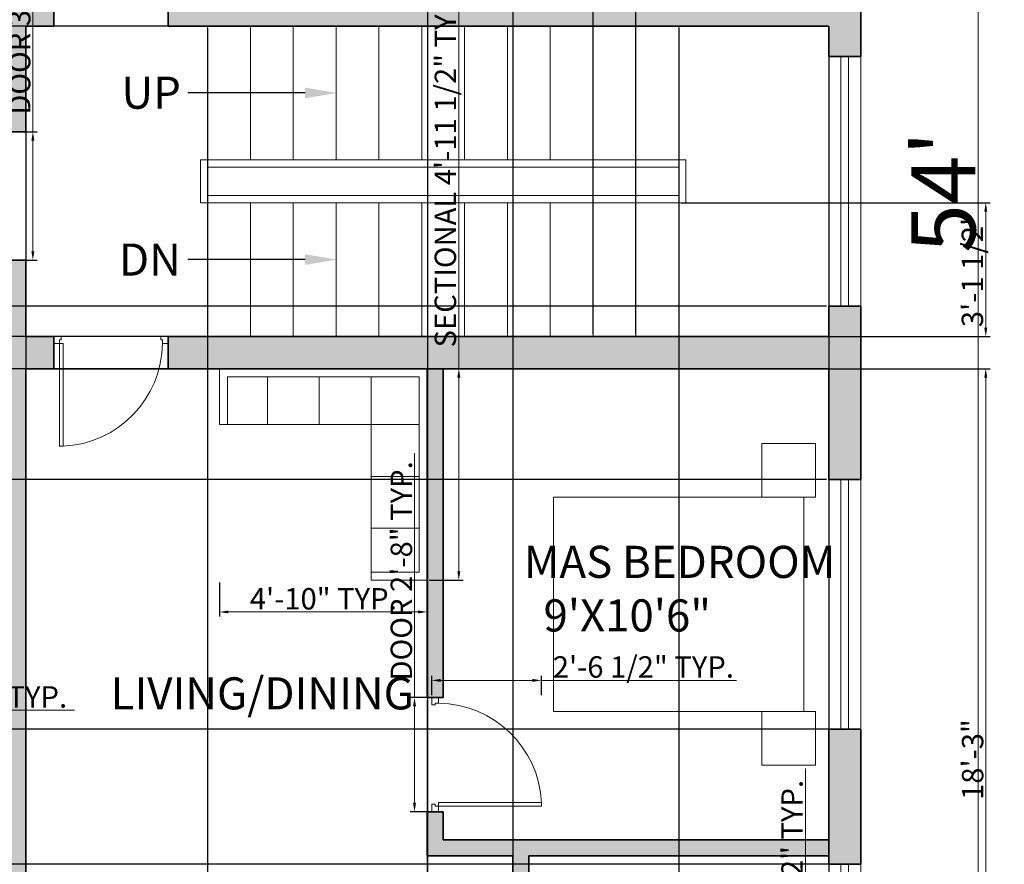
# Model space of a CAD drawing. Units: inches. Extents: x 2696 to 3240, y 1564 to 2310.
# Tile 38 of 76: x 2964 to 3240, y 1745 to 1982. Entities that reach past the tile are written whole.
import ezdxf
from ezdxf import colors
from ezdxf.entities.mleader import LeaderData, LeaderLine
from ezdxf.math import Vec2, Vec3

# ---------------------------------------------------------------- set-up
doc = ezdxf.new("R2010")
doc.units = ezdxf.units.IN
for name, color, linetype, lineweight in [('A-ANNO-DIMS', 3, 'Continuous', 18), ('A-ANNO-SYMB', 7, 'Continuous', 18), ('A-AREA-IDEN', 7, 'Continuous', 18), ('A-DOOR', 4, 'Continuous', 18), ('A-FLOR-STRS', 7, 'Continuous', 18), ('A-FURN', 251, 'Continuous', 13), ('A-WALL', 7, 'Continuous', 35), ('A-WALL-PATT', 9, 'Continuous', 13), ('WINDOW', 2, 'Continuous', 18)]:
    doc.layers.add(name, color=color, linetype=linetype, lineweight=lineweight)
doc.styles.get("Standard").update_dxf_attribs({"font": 'arial.ttf'})
doc.styles.add('TIMES NEW', font='times.ttf')
doc.styles.add('YQ_DIM', font='SUPEROS.SHX', dxfattribs={"width": 0.8, "bigfont": 'HZDX.SHX'})
doc.dimstyles.new('Siddhuu', dxfattribs={"dimtxt": 6, "dimasz": 2.5, "dimexe": 1.25, "dimexo": 0.625, "dimtad": 1, "dimdec": 1, "dimlunit": 4, "dimtxsty": 'TIMES NEW', "dimcen": 2.5, "dimclrd": 256, "dimclre": 1, "dimclrt": 7, "dimadec": 0, "dimazin": 0, "dimtfac": 1, "dimtdec": 1, "dimtmove": 0, "dimatfit": 3, "dimfxl": 1, "dimtolj": 1, "dimlwd": -1, "dimarcsym": 0})

# ---------------------------------------------------------------- blocks, each defined once
blk = doc.blocks.new('DR_D01')
for p, q in [((-0.45, 0.93), (-0.42, 0.93)), ((-0.45, 0.03), (-0.45, 0.93)), ((-0.42, 0.03), (-0.42, 0.93)), ((-0.5, 0.03), (-0.42, 0.03)), ((-0.5, 0.03), (-0.5, -0.03)), ((-0.45, 0.03), (-0.45, 0)), ((-0.45, 0), (-0.435, 0)), ((-0.435, 0), (-0.435, -0.03)), ((0.435, 0), (0.435, -0.03)), ((0.45, 0), (0.435, 0)), ((0.45, 0.03), (0.45, 0)), ((0.5, 0.03), (0.45, 0.03)), ((0.5, -0.03), (0.5, 0.03)), ((-0.435, -0.03), (-0.5, -0.03)), ((0.435, -0.03), (0.5, -0.03))]:
    blk.add_line(p, q)
blk.add_arc((-0.4602, 0.0206), 0.9103, 0.59152, 87.46644)
blk = doc.blocks.new('WD_WIN4')
for p, q in [((-0.5, 0.5), (0.5, 0.5)), ((-0.5, 0.12), (0.5, 0.12)), ((-0.5, -0.12), (0.5, -0.12)), ((-0.5, -0.5), (0.5, -0.5))]:
    blk.add_line(p, q)
blk = doc.blocks.new('*D10')
at = {"layer": 'A-ANNO-DIMS', "color": 0, "lineweight": -2, "transparency": 16777216}
for p, q in [((3200.24, 2262.2), (3233.75, 2262.2)), ((3200.24, 1605.2), (3233.75, 1605.2))]:
    blk.add_line(p, q, dxfattribs=at)
at = {"layer": 'A-ANNO-DIMS', "color": 0, "transparency": 16777216}
blk.add_line((3232.5, 2250.2), (3232.5, 1617.2), dxfattribs=at)
for points in [[(3230.5, 2250.2), (3234.5, 2250.2), (3232.5, 2262.2)], [(3230.5, 1617.2), (3234.5, 1617.2), (3232.5, 1605.2)]]:
    blk.add_solid(points, dxfattribs=at)
at = {"layer": 'Defpoints', "color": 0, "transparency": 16777216}
for p in [(3199.61, 2262.2), (3199.61, 1605.2), (3232.5, 1605.2)]:
    blk.add_point(p, dxfattribs=at)
at = {"layer": 'A-ANNO-DIMS', "color": 0, "transparency": 16777216, "insert": (3222.71, 1933.7), "char_height": 18, "attachment_point": 5, "rotation": 90, "style": 'TIMES NEW'}
blk.add_mtext("\\A1;54'", dxfattribs=at)
blk = doc.blocks.new('BED-DOUBLE-WITH-NIGHTSTANDS')
for points in [[(0, 75.13), (0, 90.16), (15.03, 90.16), (15.03, 75.13)], [(3.28, 15.03), (3.28, 75.13), (73.4, 75.13), (73.4, 15.03)], [(0, 15.03), (0, 0), (15.03, 0), (15.03, 15.03)]]:
    blk.add_lwpolyline(points, close=True)
blk = doc.blocks.new('SOFA-SECTIONAL')
for p, q in [((0, 43.61), (0, 59.26)), ((0, 59.26), (58.14, 59.26)), ((58.14, 59.26), (58.14, 0)), ((2.24, 43.61), (2.24, 57.02)), ((2.24, 57.02), (55.9, 57.02)), ((13.42, 57.02), (13.42, 43.61)), ((27.95, 57.02), (27.95, 43.61)), ((42.49, 57.02), (42.49, 0)), ((55.9, 57.02), (55.9, 2.24)), ((0, 43.61), (55.9, 43.61)), ((42.49, 29.07), (55.9, 29.07)), ((42.49, 14.54), (55.9, 14.54)), ((55.9, 2.24), (42.49, 2.24)), ((58.14, 0), (42.49, 0))]:
    blk.add_line(p, q)
blk = doc.blocks.new('*D26')
at = {"layer": 'A-ANNO-DIMS', "transparency": 16777216}
for p, q in [((3184.12, 1676.35), (3184.12, 1772.17)), ((3184.12, 1635.55), (3184.12, 1673.85))]:
    blk.add_line(p, q, dxfattribs=at)
at = {"layer": 'A-ANNO-DIMS', "color": 1, "lineweight": -2, "transparency": 16777216}
for p, q in [((3189.99, 1676.35), (3182.87, 1676.35)), ((3189.99, 1633.05), (3182.87, 1633.05))]:
    blk.add_line(p, q, dxfattribs=at)
at = {"layer": 'A-ANNO-DIMS', "transparency": 16777216}
for points in [[(3183.7, 1673.85), (3184.53, 1673.85), (3184.12, 1676.35)], [(3183.7, 1635.55), (3184.53, 1635.55), (3184.12, 1633.05)]]:
    blk.add_solid(points, dxfattribs=at)
at = {"layer": 'Defpoints', "color": 0, "transparency": 16777216}
for p in [(3184.12, 1676.35), (3190.61, 1676.35), (3190.61, 1633.05)]:
    blk.add_point(p, dxfattribs=at)
at = {"layer": 'A-ANNO-DIMS', "color": 7, "transparency": 16777216, "insert": (3180.35, 1725.51), "char_height": 6, "attachment_point": 5, "rotation": 90, "style": 'TIMES NEW'}
blk.add_mtext('\\A1;WINDOW 3\'-7 1/2" TYP.', dxfattribs=at)
blk = doc.blocks.new('*D30')
at = {"layer": 'A-ANNO-DIMS', "transparency": 16777216}
for p, q in [((2967.69, 1950.58), (2967.69, 2019.05)), ((2967.69, 1917.08), (2967.69, 1948.08))]:
    blk.add_line(p, q, dxfattribs=at)
at = {"layer": 'A-ANNO-DIMS', "color": 1, "lineweight": -2, "transparency": 16777216}
for p, q in [((2962.91, 1950.58), (2968.94, 1950.58)), ((2962.91, 1914.58), (2968.94, 1914.58))]:
    blk.add_line(p, q, dxfattribs=at)
at = {"layer": 'A-ANNO-DIMS', "transparency": 16777216}
for points in [[(2967.27, 1948.08), (2968.11, 1948.08), (2967.69, 1950.58)], [(2967.27, 1917.08), (2968.11, 1917.08), (2967.69, 1914.58)]]:
    blk.add_solid(points, dxfattribs=at)
at = {"layer": 'Defpoints', "color": 0, "transparency": 16777216}
for p in [(2962.29, 1950.58), (2967.69, 1950.58), (2962.29, 1914.58)]:
    blk.add_point(p, dxfattribs=at)
at = {"layer": 'A-ANNO-DIMS', "color": 7, "transparency": 16777216, "insert": (2964, 1986.06), "char_height": 6, "attachment_point": 5, "rotation": 90, "style": 'TIMES NEW'}
blk.add_mtext('\\A1;DOOR 3\'-0" TYP.', dxfattribs=at)
blk = doc.blocks.new('*D34')
at = {"layer": 'A-ANNO-DIMS', "transparency": 16777216}
for p, q in [((3074.6, 1792.08), (3074.6, 1860.55)), ((3074.6, 1762.58), (3074.6, 1789.58))]:
    blk.add_line(p, q, dxfattribs=at)
at = {"layer": 'A-ANNO-DIMS', "color": 1, "lineweight": -2, "transparency": 16777216}
for p, q in [((3078.78, 1792.08), (3073.35, 1792.08)), ((3078.78, 1760.08), (3073.35, 1760.08))]:
    blk.add_line(p, q, dxfattribs=at)
at = {"layer": 'A-ANNO-DIMS', "transparency": 16777216}
for points in [[(3074.18, 1789.58), (3075.02, 1789.58), (3074.6, 1792.08)], [(3074.18, 1762.58), (3075.02, 1762.58), (3074.6, 1760.08)]]:
    blk.add_solid(points, dxfattribs=at)
at = {"layer": 'Defpoints', "color": 0, "transparency": 16777216}
for p in [(3074.6, 1792.08), (3079.4, 1792.08), (3079.4, 1760.08)]:
    blk.add_point(p, dxfattribs=at)
at = {"layer": 'A-ANNO-DIMS', "color": 7, "transparency": 16777216, "insert": (3070.91, 1827.56), "char_height": 6, "attachment_point": 5, "rotation": 90, "style": 'TIMES NEW'}
blk.add_mtext('\\A1;DOOR 2\'-8" TYP.', dxfattribs=at)
blk = doc.blocks.new('*D35')
at = {"layer": 'A-ANNO-DIMS', "color": 1, "lineweight": -2, "transparency": 16777216}
for p, q in [((3079.4, 1792.7), (3079.4, 1798.13)), ((3110.12, 1792.7), (3110.12, 1798.13))]:
    blk.add_line(p, q, dxfattribs=at)
at = {"layer": 'A-ANNO-DIMS', "transparency": 16777216}
for p, q in [((3081.9, 1796.88), (3107.62, 1796.88)), ((3110.12, 1796.88), (3164.78, 1796.88))]:
    blk.add_line(p, q, dxfattribs=at)
for points in [[(3081.9, 1797.29), (3081.9, 1796.46), (3079.4, 1796.88)], [(3107.62, 1797.29), (3107.62, 1796.46), (3110.12, 1796.88)]]:
    blk.add_solid(points, dxfattribs=at)
at = {"layer": 'Defpoints', "color": 0, "transparency": 16777216}
for p in [(3110.12, 1796.88), (3079.4, 1792.08), (3110.12, 1792.08)]:
    blk.add_point(p, dxfattribs=at)
at = {"layer": 'A-ANNO-DIMS', "color": 7, "transparency": 16777216, "insert": (3138.7, 1800.64), "char_height": 6, "attachment_point": 5, "style": 'TIMES NEW'}
blk.add_mtext('\\A1;2\'-6 1/2" TYP.', dxfattribs=at)
blk = doc.blocks.new('*D42')
at = {"layer": 'A-ANNO-DIMS', "color": 1, "lineweight": -2, "transparency": 16777216}
for p, q in [((2884.71, 1792.59), (2884.71, 1787.31)), ((2915.75, 1792.59), (2915.75, 1787.31))]:
    blk.add_line(p, q, dxfattribs=at)
at = {"layer": 'A-ANNO-DIMS', "transparency": 16777216}
for p, q in [((2887.21, 1788.56), (2913.25, 1788.56)), ((2915.75, 1788.56), (2979.39, 1788.56))]:
    blk.add_line(p, q, dxfattribs=at)
for points in [[(2887.21, 1788.98), (2887.21, 1788.14), (2884.71, 1788.56)], [(2913.25, 1788.98), (2913.25, 1788.14), (2915.75, 1788.56)]]:
    blk.add_solid(points, dxfattribs=at)
at = {"layer": 'Defpoints', "color": 0, "transparency": 16777216}
for p in [(2884.71, 1793.22), (2915.75, 1793.22), (2915.75, 1788.56)]:
    blk.add_point(p, dxfattribs=at)
at = {"layer": 'A-ANNO-DIMS', "color": 7, "transparency": 16777216, "insert": (2948.82, 1792.25), "char_height": 6, "attachment_point": 5, "style": 'TIMES NEW'}
blk.add_mtext('\\A1;SINK 2\'-7" TYP.', dxfattribs=at)
blk = doc.blocks.new('*D48')
at = {"layer": 'A-ANNO-DIMS', "transparency": 16777216}
for p, q in [((3087, 1884.2), (3087, 1994.35)), ((3087, 1827.44), (3087, 1881.7))]:
    blk.add_line(p, q, dxfattribs=at)
at = {"layer": 'A-ANNO-DIMS', "color": 1, "lineweight": -2, "transparency": 16777216}
for p, q in [((3078.74, 1884.2), (3088.25, 1884.2)), ((3078.74, 1824.94), (3088.25, 1824.94))]:
    blk.add_line(p, q, dxfattribs=at)
at = {"layer": 'A-ANNO-DIMS', "transparency": 16777216}
for points in [[(3086.58, 1881.7), (3087.42, 1881.7), (3087, 1884.2)], [(3086.58, 1827.44), (3087.42, 1827.44), (3087, 1824.94)]]:
    blk.add_solid(points, dxfattribs=at)
at = {"layer": 'Defpoints', "color": 0, "transparency": 16777216}
for p in [(3078.11, 1884.2), (3087, 1884.2), (3078.11, 1824.94)]:
    blk.add_point(p, dxfattribs=at)
at = {"layer": 'A-ANNO-DIMS', "color": 7, "transparency": 16777216, "insert": (3083.23, 1940.53), "char_height": 6, "attachment_point": 5, "rotation": 90, "style": 'TIMES NEW'}
blk.add_mtext('\\A1;SECTIONAL 4\'-11 1/2" TYP.', dxfattribs=at)
blk = doc.blocks.new('*D49')
at = {"layer": 'A-ANNO-DIMS', "color": 1, "lineweight": -2, "transparency": 16777216}
for p, q in [((3019.97, 1824.32), (3019.97, 1814.8)), ((3078.11, 1824.32), (3078.11, 1814.8))]:
    blk.add_line(p, q, dxfattribs=at)
at = {"layer": 'A-ANNO-DIMS', "transparency": 16777216}
blk.add_line((3022.47, 1816.05), (3075.61, 1816.05), dxfattribs=at)
for points in [[(3022.47, 1816.47), (3022.47, 1815.64), (3019.97, 1816.05)], [(3075.61, 1816.47), (3075.61, 1815.64), (3078.11, 1816.05)]]:
    blk.add_solid(points, dxfattribs=at)
at = {"layer": 'Defpoints', "color": 0, "transparency": 16777216}
for p in [(3019.97, 1824.94), (3078.11, 1824.94), (3078.11, 1816.05)]:
    blk.add_point(p, dxfattribs=at)
at = {"layer": 'A-ANNO-DIMS', "color": 7, "transparency": 16777216, "insert": (3049.04, 1819.74), "char_height": 6, "attachment_point": 5, "style": 'TIMES NEW'}
blk.add_mtext('\\A1;4\'-10" TYP.', dxfattribs=at)
blk = doc.blocks.new('*D50')
at = {"layer": 'A-ANNO-DIMS', "color": 1, "lineweight": -2, "transparency": 16777216}
for p, q in [((2965.71, 1979.58), (2965.71, 1568.95)), ((3016.61, 1979.58), (3016.61, 1568.95))]:
    blk.add_line(p, q, dxfattribs=at)
at = {"layer": 'A-ANNO-DIMS', "transparency": 16777216}
blk.add_line((2968.21, 1570.2), (3014.11, 1570.2), dxfattribs=at)
for points in [[(2968.21, 1570.62), (2968.21, 1569.78), (2965.71, 1570.2)], [(3014.11, 1570.62), (3014.11, 1569.78), (3016.61, 1570.2)]]:
    blk.add_solid(points, dxfattribs=at)
at = {"layer": 'Defpoints', "color": 0, "transparency": 16777216}
for p in [(2965.71, 1980.2), (3016.61, 1980.2), (3016.61, 1570.2)]:
    blk.add_point(p, dxfattribs=at)
at = {"layer": 'A-ANNO-DIMS', "color": 7, "transparency": 16777216, "insert": (2991.16, 1573.88), "char_height": 6, "attachment_point": 5, "style": 'TIMES NEW'}
blk.add_mtext('\\A1;4\'-3"', dxfattribs=at)
blk = doc.blocks.new('*D51')
at = {"layer": 'A-ANNO-DIMS', "color": 1, "lineweight": -2, "transparency": 16777216}
for p, q in [((3016.61, 1979.58), (3016.61, 1568.95)), ((3148.61, 1979.58), (3148.61, 1568.95))]:
    blk.add_line(p, q, dxfattribs=at)
at = {"layer": 'A-ANNO-DIMS', "transparency": 16777216}
blk.add_line((3019.11, 1570.2), (3146.11, 1570.2), dxfattribs=at)
for points in [[(3019.11, 1570.62), (3019.11, 1569.78), (3016.61, 1570.2)], [(3146.11, 1570.62), (3146.11, 1569.78), (3148.61, 1570.2)]]:
    blk.add_solid(points, dxfattribs=at)
at = {"layer": 'Defpoints', "color": 0, "transparency": 16777216}
for p in [(3016.61, 1980.2), (3148.61, 1980.2), (3148.61, 1570.2)]:
    blk.add_point(p, dxfattribs=at)
at = {"layer": 'A-ANNO-DIMS', "color": 7, "transparency": 16777216, "insert": (3082.61, 1573.88), "char_height": 6, "attachment_point": 5, "style": 'TIMES NEW'}
blk.add_mtext('\\A1;11\'-0"', dxfattribs=at)
blk = doc.blocks.new('*D52')
at = {"layer": 'A-ANNO-DIMS', "color": 1, "lineweight": -2, "transparency": 16777216}
for p, q in [((3148.61, 1979.58), (3148.61, 1568.95)), ((3190.61, 1979.58), (3190.61, 1568.95))]:
    blk.add_line(p, q, dxfattribs=at)
at = {"layer": 'A-ANNO-DIMS', "transparency": 16777216}
blk.add_line((3151.11, 1570.2), (3188.11, 1570.2), dxfattribs=at)
for points in [[(3151.11, 1570.62), (3151.11, 1569.78), (3148.61, 1570.2)], [(3188.11, 1570.62), (3188.11, 1569.78), (3190.61, 1570.2)]]:
    blk.add_solid(points, dxfattribs=at)
at = {"layer": 'Defpoints', "color": 0, "transparency": 16777216}
for p in [(3148.61, 1980.2), (3190.61, 1980.2), (3190.61, 1570.2)]:
    blk.add_point(p, dxfattribs=at)
at = {"layer": 'A-ANNO-DIMS', "color": 7, "transparency": 16777216, "insert": (3169.61, 1573.88), "char_height": 6, "attachment_point": 5, "style": 'TIMES NEW'}
blk.add_mtext('\\A1;3\'-6"', dxfattribs=at)
blk = doc.blocks.new('*D53')
at = {"layer": 'A-ANNO-DIMS', "color": 1, "lineweight": -2, "transparency": 16777216}
for p, q in [((3149.24, 1930.7), (3235.86, 1930.7)), ((3149.24, 1893.2), (3235.86, 1893.2))]:
    blk.add_line(p, q, dxfattribs=at)
at = {"layer": 'A-ANNO-DIMS', "transparency": 16777216}
blk.add_line((3234.61, 1895.7), (3234.61, 1928.2), dxfattribs=at)
for points in [[(3234.19, 1928.2), (3235.03, 1928.2), (3234.61, 1930.7)], [(3234.19, 1895.7), (3235.03, 1895.7), (3234.61, 1893.2)]]:
    blk.add_solid(points, dxfattribs=at)
at = {"layer": 'Defpoints', "color": 0, "transparency": 16777216}
for p in [(3148.61, 1930.7), (3234.61, 1930.7), (3148.61, 1893.2)]:
    blk.add_point(p, dxfattribs=at)
at = {"layer": 'A-ANNO-DIMS', "color": 7, "transparency": 16777216, "insert": (3230.85, 1911.95), "char_height": 6, "attachment_point": 5, "rotation": 90, "style": 'TIMES NEW'}
blk.add_mtext('\\A1;3\'-1 1/2"', dxfattribs=at)
blk = doc.blocks.new('*D54')
at = {"layer": 'A-ANNO-DIMS', "color": 1, "lineweight": -2, "transparency": 16777216}
for p, q in [((3124.61, 1893.83), (3124.61, 2298.45)), ((3136.61, 1893.83), (3136.61, 2298.45))]:
    blk.add_line(p, q, dxfattribs=at)
at = {"layer": 'A-ANNO-DIMS', "transparency": 16777216}
for p, q in [((3127.11, 2297.2), (3134.11, 2297.2)), ((3136.61, 2297.2), (3155.76, 2297.2))]:
    blk.add_line(p, q, dxfattribs=at)
for points in [[(3127.11, 2297.62), (3127.11, 2296.78), (3124.61, 2297.2)], [(3134.11, 2297.62), (3134.11, 2296.78), (3136.61, 2297.2)]]:
    blk.add_solid(points, dxfattribs=at)
at = {"layer": 'Defpoints', "color": 0, "transparency": 16777216}
for p in [(3136.61, 2297.2), (3124.61, 1893.2), (3136.61, 1893.2)]:
    blk.add_point(p, dxfattribs=at)
at = {"layer": 'A-ANNO-DIMS', "color": 7, "transparency": 16777216, "insert": (3147.43, 2300.88), "char_height": 6, "attachment_point": 5, "style": 'TIMES NEW'}
blk.add_mtext('\\A1;1\'-0"', dxfattribs=at)
blk = doc.blocks.new('*D55')
at = {"layer": 'A-ANNO-DIMS', "color": 1, "lineweight": -2, "transparency": 16777216}
for p, q in [((3189.99, 1980.2), (2709.36, 1980.2)), ((3189.99, 1893.2), (2709.36, 1893.2))]:
    blk.add_line(p, q, dxfattribs=at)
at = {"layer": 'A-ANNO-DIMS', "transparency": 16777216}
blk.add_line((2710.61, 1895.7), (2710.61, 1977.7), dxfattribs=at)
for points in [[(2710.19, 1977.7), (2711.03, 1977.7), (2710.61, 1980.2)], [(2710.19, 1895.7), (2711.03, 1895.7), (2710.61, 1893.2)]]:
    blk.add_solid(points, dxfattribs=at)
at = {"layer": 'Defpoints', "color": 0, "transparency": 16777216}
for p in [(2710.61, 1980.2), (3190.61, 1980.2), (3190.61, 1893.2)]:
    blk.add_point(p, dxfattribs=at)
at = {"layer": 'A-ANNO-DIMS', "color": 7, "transparency": 16777216, "insert": (2706.93, 1936.7), "char_height": 6, "attachment_point": 5, "rotation": 90, "style": 'TIMES NEW'}
blk.add_mtext('\\A1;7\'-3"', dxfattribs=at)
blk = doc.blocks.new('*D56')
at = {"layer": 'A-ANNO-DIMS', "color": 1, "lineweight": -2, "transparency": 16777216}
for p, q in [((2966.33, 1884.2), (3235.86, 1884.2)), ((2966.33, 1665.2), (3235.86, 1665.2))]:
    blk.add_line(p, q, dxfattribs=at)
at = {"layer": 'A-ANNO-DIMS', "transparency": 16777216}
blk.add_line((3234.61, 1667.7), (3234.61, 1881.7), dxfattribs=at)
for points in [[(3234.19, 1881.7), (3235.03, 1881.7), (3234.61, 1884.2)], [(3234.19, 1667.7), (3235.03, 1667.7), (3234.61, 1665.2)]]:
    blk.add_solid(points, dxfattribs=at)
at = {"layer": 'Defpoints', "color": 0, "transparency": 16777216}
for p in [(2965.71, 1884.2), (3234.61, 1884.2), (2965.71, 1665.2)]:
    blk.add_point(p, dxfattribs=at)
at = {"layer": 'A-ANNO-DIMS', "color": 7, "transparency": 16777216, "insert": (3230.93, 1774.7), "char_height": 6, "attachment_point": 5, "rotation": 90, "style": 'TIMES NEW'}
blk.add_mtext('\\A1;18\'-3"', dxfattribs=at)
blk = doc.blocks.new('*D65')
at = {"layer": 'A-ANNO-DIMS', "color": 1, "lineweight": -2, "transparency": 16777216}
for p, q in [((3078.21, 2122.08), (3078.21, 1568.95)), ((3102.11, 2122.08), (3102.11, 1568.95))]:
    blk.add_line(p, q, dxfattribs=at)
at = {"layer": 'A-ANNO-DIMS', "transparency": 16777216}
blk.add_line((3080.71, 1570.2), (3099.61, 1570.2), dxfattribs=at)
for points in [[(3080.71, 1570.62), (3080.71, 1569.78), (3078.21, 1570.2)], [(3099.61, 1570.62), (3099.61, 1569.78), (3102.11, 1570.2)]]:
    blk.add_solid(points, dxfattribs=at)
at = {"layer": 'Defpoints', "color": 0, "transparency": 16777216}
for p in [(3078.21, 2122.7), (3102.11, 2122.7), (3102.11, 1570.2)]:
    blk.add_point(p, dxfattribs=at)
at = {"layer": 'A-ANNO-DIMS', "color": 7, "transparency": 16777216, "insert": (3090.16, 1573.88), "char_height": 6, "attachment_point": 5, "style": 'TIMES NEW'}
blk.add_mtext('\\A1;2\'-0"', dxfattribs=at)
blk = doc.blocks.new('*D67')
at = {"layer": 'A-ANNO-DIMS', "color": 1, "lineweight": -2, "transparency": 16777216}
for p, q in [((2965.71, 1883.58), (2965.71, 1568.95)), ((3078.11, 1791.45), (3078.11, 1568.95))]:
    blk.add_line(p, q, dxfattribs=at)
at = {"layer": 'A-ANNO-DIMS', "transparency": 16777216}
blk.add_line((2968.21, 1570.2), (3075.61, 1570.2), dxfattribs=at)
for points in [[(2968.21, 1570.62), (2968.21, 1569.78), (2965.71, 1570.2)], [(3075.61, 1570.62), (3075.61, 1569.78), (3078.11, 1570.2)]]:
    blk.add_solid(points, dxfattribs=at)
at = {"layer": 'Defpoints', "color": 0, "transparency": 16777216}
for p in [(2965.71, 1884.2), (3078.11, 1792.08), (3078.11, 1570.2)]:
    blk.add_point(p, dxfattribs=at)
at = {"layer": 'A-ANNO-DIMS', "color": 7, "transparency": 16777216, "insert": (3021.91, 1573.96), "char_height": 6, "attachment_point": 5, "style": 'TIMES NEW'}
blk.add_mtext('\\A1;9\'-4 1/2"', dxfattribs=at)
blk = doc.blocks.new('*D78')
at = {"layer": 'A-ANNO-DIMS', "transparency": 16777216}
for p, q in [((2710.61, 1901.7), (2710.61, 1935.1)), ((2710.61, 1895.7), (2710.61, 1899.2))]:
    blk.add_line(p, q, dxfattribs=at)
at = {"layer": 'A-ANNO-DIMS', "color": 1, "lineweight": -2, "transparency": 16777216}
for p, q in [((3189.99, 1901.7), (2709.36, 1901.7)), ((3189.99, 1893.2), (2709.36, 1893.2))]:
    blk.add_line(p, q, dxfattribs=at)
at = {"layer": 'A-ANNO-DIMS', "transparency": 16777216}
for points in [[(2710.19, 1899.2), (2711.03, 1899.2), (2710.61, 1901.7)], [(2710.19, 1895.7), (2711.03, 1895.7), (2710.61, 1893.2)]]:
    blk.add_solid(points, dxfattribs=at)
at = {"layer": 'Defpoints', "color": 0, "transparency": 16777216}
for p in [(2710.61, 1901.7), (3190.61, 1901.7), (3190.61, 1893.2)]:
    blk.add_point(p, dxfattribs=at)
at = {"layer": 'A-ANNO-DIMS', "color": 7, "transparency": 16777216, "insert": (2706.85, 1919.65), "char_height": 6, "attachment_point": 5, "rotation": 90, "style": 'TIMES NEW'}
blk.add_mtext('\\A1;0\'-8 1/2"', dxfattribs=at)
blk = doc.blocks.new('*D79')
at = {"layer": 'A-ANNO-DIMS', "color": 1, "lineweight": -2, "transparency": 16777216}
for p, q in [((3189.99, 1884.2), (2709.36, 1884.2)), ((3189.99, 1853.2), (2709.36, 1853.2))]:
    blk.add_line(p, q, dxfattribs=at)
at = {"layer": 'A-ANNO-DIMS', "transparency": 16777216}
blk.add_line((2710.61, 1881.7), (2710.61, 1855.7), dxfattribs=at)
for points in [[(2710.19, 1881.7), (2711.03, 1881.7), (2710.61, 1884.2)], [(2710.19, 1855.7), (2711.03, 1855.7), (2710.61, 1853.2)]]:
    blk.add_solid(points, dxfattribs=at)
at = {"layer": 'Defpoints', "color": 0, "transparency": 16777216}
for p in [(3190.61, 1884.2), (2710.61, 1853.2), (3190.61, 1853.2)]:
    blk.add_point(p, dxfattribs=at)
at = {"layer": 'A-ANNO-DIMS', "color": 7, "transparency": 16777216, "insert": (2706.93, 1868.7), "char_height": 6, "attachment_point": 5, "rotation": 90, "style": 'TIMES NEW'}
blk.add_mtext('\\A1;2\'-7"', dxfattribs=at)
blk = doc.blocks.new('*D80')
at = {"layer": 'A-ANNO-DIMS', "color": 1, "lineweight": -2, "transparency": 16777216}
for p, q in [((3198.99, 1783.2), (2709.36, 1783.2)), ((3198.99, 1745.35), (2709.36, 1745.35))]:
    blk.add_line(p, q, dxfattribs=at)
at = {"layer": 'A-ANNO-DIMS', "transparency": 16777216}
blk.add_line((2710.61, 1780.7), (2710.61, 1747.85), dxfattribs=at)
for points in [[(2710.19, 1780.7), (2711.03, 1780.7), (2710.61, 1783.2)], [(2710.19, 1747.85), (2711.03, 1747.85), (2710.61, 1745.35)]]:
    blk.add_solid(points, dxfattribs=at)
at = {"layer": 'Defpoints', "color": 0, "transparency": 16777216}
for p in [(3199.61, 1783.2), (2710.61, 1745.35), (3199.61, 1745.35)]:
    blk.add_point(p, dxfattribs=at)
at = {"layer": 'A-ANNO-DIMS', "color": 7, "transparency": 16777216, "insert": (2706.93, 1764.28), "char_height": 6, "attachment_point": 5, "rotation": 90, "style": 'TIMES NEW'}
blk.add_mtext('\\A1;3\'-2"', dxfattribs=at)

msp = doc.modelspace()

# ---------------------------------------------------------------- hatches: boundary and pattern name
at = {"layer": 'A-WALL-PATT', "transparency": 33554556}
h = msp.add_hatch(color=256, dxfattribs=at)
h.dxf.hatch_style = 1
h.paths.add_polyline_path([(2879.11, 2253.2), (2905.91, 2253.2), (2905.91, 2262.2), (2841.89, 2262.2), (2841.89, 2253.2), (2870.11, 2253.2), (2870.11, 2176.6), (2965.71, 2176.6), (2965.71, 2206.7), (2973.58, 2206.7), (2973.58, 2215.7), (2965.71, 2215.7), (2965.71, 2262.2), (2929.91, 2262.2), (2929.91, 2253.2), (2956.71, 2253.2), (2956.71, 2185.6), (2879.11, 2185.6)])
h.paths.add_polyline_path([(2782.83, 2262.2), (2745.61, 2262.2), (2745.61, 2228.73), (2754.61, 2228.73), (2754.61, 2253.2), (2782.83, 2253.2)])
h.paths.add_polyline_path([(2754.61, 2136.2), (2965.71, 2136.2), (2965.71, 2145.2), (2879.11, 2145.2), (2879.11, 2147.07), (2877.34, 2147.07), (2870.11, 2147.07), (2870.11, 2145.2), (2754.61, 2145.2), (2754.61, 2169.67), (2745.61, 2169.67), (2745.61, 2000.2), (2754.61, 2000.2), (2754.61, 2019.2), (2849.08, 2019.2), (2849.08, 2023.7), (2841.21, 2023.7), (2841.21, 2051.83), (2836.71, 2051.83), (2836.71, 2023.7), (2754.61, 2023.7), (2754.61, 2091.2), (2836.71, 2091.2), (2836.71, 2087.83), (2841.21, 2087.83), (2841.21, 2095.7), (2754.61, 2095.7)])
h.paths.add_polyline_path([(2965.71, 2136.2), (2956.71, 2136.2), (2956.71, 2023.7), (2885.08, 2023.7), (2885.08, 2019.2), (2956.71, 2019.2), (2956.71, 1950.58), (2965.71, 1950.58), (2965.71, 1980.2), (2973.58, 1980.2), (2973.58, 1989.2), (2965.71, 1989.2)])
h.paths.add_polyline_path([(2754.61, 1906.7), (2880.21, 1906.7), (2884.71, 1906.7), (2956.71, 1906.7), (2956.71, 1792.7), (2944.71, 1792.7), (2944.71, 1783.7), (2956.71, 1783.7), (2956.71, 1740.2), (2884.71, 1740.2), (2884.71, 1783.7), (2896.71, 1783.7), (2896.71, 1792.7), (2884.71, 1792.7), (2884.71, 1846.7), (2880.21, 1846.7), (2880.21, 1740.2), (2754.61, 1740.2), (2754.61, 1777.2), (2745.61, 1777.2), (2745.61, 1692.7), (2754.61, 1692.7), (2754.61, 1731.2), (2956.71, 1731.2), (2956.71, 1723.33), (2965.71, 1723.33), (2965.71, 1884.2), (2973.58, 1884.2), (2973.58, 1893.2), (2965.71, 1893.2), (2965.71, 1914.58), (2956.71, 1914.58), (2956.71, 1911.2), (2754.61, 1911.2), (2754.61, 1930.2), (2745.61, 1930.2), (2745.61, 1817.2), (2754.61, 1817.2), (2754.61, 1854.2), (2826.61, 1854.2), (2826.61, 1868.83), (2822.11, 1868.83), (2822.11, 1858.7), (2754.61, 1858.7)])
h.paths.add_polyline_path([(2965.71, 1656.2), (3008.24, 1656.2), (3008.24, 1665.2), (2965.71, 1665.2), (2965.71, 1693.33), (2956.71, 1693.33), (2956.71, 1686.2), (2934.58, 1686.2), (2934.58, 1681.7), (2956.71, 1681.7), (2956.71, 1614.2), (2896.71, 1614.2), (2896.71, 1681.7), (2904.58, 1681.7), (2904.58, 1686.2), (2892.21, 1686.2), (2892.21, 1614.2), (2858.41, 1614.2), (2858.41, 1605.2), (2965.71, 1605.2)])
h.paths.add_polyline_path([(2788.41, 1614.2), (2754.61, 1614.2), (2754.61, 1652.7), (2745.61, 1652.7), (2745.61, 1605.2), (2788.41, 1605.2)])
h.paths.add_polyline_path([(3199.61, 1633.05), (3190.61, 1633.05), (3190.61, 1614.2), (3082.61, 1614.2), (3082.61, 1665.2), (3070.24, 1665.2), (3070.24, 1656.2), (3078.11, 1656.2), (3078.11, 1605.2), (3199.61, 1605.2)])
h.paths.add_polyline_path([(3199.61, 1702.05), (3190.61, 1702.05), (3190.61, 1699.7), (3106.61, 1699.7), (3106.61, 1747.7), (3190.61, 1747.7), (3190.61, 1752.2), (3082.61, 1752.2), (3082.61, 1760.08), (3078.11, 1760.08), (3078.11, 1747.7), (3102.11, 1747.7), (3102.11, 1699.7), (3078.11, 1699.7), (3078.11, 1695.2), (3190.61, 1695.2), (3190.61, 1676.35), (3199.61, 1676.35)])
h.paths.add_polyline_path([(3199.61, 1783.2), (3190.61, 1783.2), (3190.61, 1745.35), (3199.61, 1745.35)])
h.paths.add_polyline_path([(3082.61, 1884.2), (3190.61, 1884.2), (3190.61, 1853.2), (3199.61, 1853.2), (3199.61, 1901.7), (3190.61, 1901.7), (3190.61, 1893.2), (3005.58, 1893.2), (3005.58, 1891.28), (3005.58, 1884.2), (3078.11, 1884.2), (3078.11, 1792.08), (3082.61, 1792.08)])
h.paths.add_polyline_path([(3199.61, 1994.7), (3190.61, 1994.7), (3190.61, 1989.2), (3073.71, 1989.2), (3073.71, 2034.2), (3069.21, 2034.2), (3069.21, 1989.2), (3005.58, 1989.2), (3005.58, 1980.2), (3190.61, 1980.2), (3190.61, 1971.7), (3199.61, 1971.7)])
h.paths.add_polyline_path([(3199.61, 2155.2), (3190.61, 2155.2), (3190.61, 2064.7), (3199.61, 2064.7)])
h.paths.add_polyline_path([(3190.61, 2074.7), (3106.61, 2074.7), (3106.61, 2122.7), (3190.61, 2122.7), (3190.61, 2127.2), (3082.71, 2127.2), (3082.71, 2135.08), (3073.71, 2135.08), (3073.71, 2122.7), (3102.11, 2122.7), (3102.11, 2074.7), (3069.21, 2074.7), (3069.21, 2070.2), (3190.61, 2070.2)])
h.paths.add_polyline_path([(3082.71, 2253.2), (3190.61, 2253.2), (3190.61, 2225.2), (3199.61, 2225.2), (3199.61, 2262.2), (3073.71, 2262.2), (3073.71, 2215.7), (3035.58, 2215.7), (3035.58, 2206.7), (3073.71, 2206.7), (3073.71, 2171.08), (3082.71, 2171.08)])

# ---------------------------------------------------------------- linework, layer by layer
at = {"layer": 'A-FLOR-STRS'}
for p, q in [((3016.61, 1942.7), (3016.61, 1980.2)), ((3028.61, 1942.7), (3028.61, 1980.2)), ((3040.61, 1942.7), (3040.61, 1980.2)), ((3052.61, 1942.7), (3052.61, 1980.2)), ((3064.61, 1942.7), (3064.61, 1980.2)), ((3076.61, 1942.7), (3076.61, 1980.2)), ((3088.61, 1942.7), (3088.61, 1980.2)), ((3100.61, 1942.7), (3100.61, 1980.2)), ((3112.61, 1942.7), (3112.61, 1980.2)), ((3124.61, 1942.7), (3124.61, 1980.2)), ((3136.61, 1942.7), (3136.61, 1980.2)), ((3148.61, 1942.7), (3148.61, 1980.2)), ((3014.61, 1942.7), (3150.61, 1942.7)), ((3014.61, 1930.7), (3014.61, 1942.7)), ((3150.61, 1930.7), (3150.61, 1942.7)), ((3016.61, 1940.7), (3148.61, 1940.7)), ((3016.61, 1932.7), (3016.61, 1940.7)), ((3148.61, 1932.7), (3148.61, 1940.7)), ((3014.61, 1930.7), (3150.61, 1930.7)), ((3016.61, 1932.7), (3148.61, 1932.7)), ((3016.61, 1893.2), (3016.61, 1930.7)), ((3028.61, 1893.2), (3028.61, 1930.7)), ((3040.61, 1893.2), (3040.61, 1930.7)), ((3052.61, 1893.2), (3052.61, 1930.7)), ((3064.61, 1893.2), (3064.61, 1930.7)), ((3076.61, 1893.2), (3076.61, 1930.7)), ((3088.61, 1893.2), (3088.61, 1930.7)), ((3100.61, 1893.2), (3100.61, 1930.7)), ((3112.61, 1893.2), (3112.61, 1930.7)), ((3124.61, 1893.2), (3124.61, 1930.7)), ((3136.61, 1893.2), (3136.61, 1930.7)), ((3148.61, 1893.2), (3148.61, 1930.7))]:
    msp.add_line(p, q, dxfattribs=at)
at = {"layer": 'A-WALL'}
for p, q in [((3199.61, 1971.7), (3199.61, 1994.7)), ((2973.58, 1980.2), (2973.58, 1989.2)), ((3005.58, 1980.2), (3005.58, 1989.2)), ((2965.71, 1980.2), (2973.58, 1980.2)), ((2965.71, 1980.2), (2965.71, 1950.58)), ((3005.58, 1980.2), (3190.61, 1980.2)), ((3190.61, 1971.7), (3190.61, 1980.2)), ((3190.61, 1971.7), (3199.61, 1971.7)), ((2965.71, 1950.58), (2956.71, 1950.58)), ((2965.71, 1914.58), (2956.71, 1914.58)), ((2965.71, 1914.58), (2965.71, 1893.2)), ((3190.61, 1893.2), (3190.61, 1901.7)), ((3190.61, 1901.7), (3199.61, 1901.7)), ((3199.61, 1853.2), (3199.61, 1901.7)), ((2965.71, 1893.2), (2973.58, 1893.2)), ((2973.58, 1893.2), (2973.58, 1884.2)), ((3005.58, 1893.2), (3190.61, 1893.2)), ((3005.58, 1893.2), (3005.58, 1884.2)), ((2965.71, 1884.2), (2973.58, 1884.2)), ((2965.71, 1884.2), (2965.71, 1723.33)), ((3005.58, 1884.2), (3078.11, 1884.2)), ((3078.11, 1792.08), (3078.11, 1884.2)), ((3082.61, 1792.08), (3082.61, 1884.2)), ((3082.61, 1884.2), (3190.61, 1884.2)), ((3190.61, 1853.2), (3190.61, 1884.2)), ((3190.61, 1853.2), (3199.61, 1853.2)), ((3082.61, 1792.08), (3078.11, 1792.08)), ((3190.61, 1783.2), (3199.61, 1783.2)), ((3190.61, 1745.35), (3190.61, 1783.2)), ((3199.61, 1745.35), (3199.61, 1783.2)), ((3078.11, 1747.7), (3078.11, 1760.08)), ((3082.61, 1760.08), (3078.11, 1760.08)), ((3082.61, 1752.2), (3082.61, 1760.08)), ((3082.61, 1752.2), (3190.61, 1752.2)), ((3078.11, 1747.7), (3102.11, 1747.7)), ((3102.11, 1699.7), (3102.11, 1747.7)), ((3106.61, 1699.7), (3106.61, 1747.7)), ((3106.61, 1747.7), (3190.61, 1747.7)), ((3190.61, 1745.35), (3199.61, 1745.35))]:
    msp.add_line(p, q, dxfattribs=at)

# ---------------------------------------------------------------- block references
at = {"layer": 'A-DOOR', "xscale": 32, "yscale": -32, "zscale": 32}
msp.add_blockref('DR_D01', (2989.58, 1892.24), dxfattribs=at)
at = {"layer": 'A-DOOR', "xscale": 32, "yscale": -32, "zscale": 32, "rotation": 90}
msp.add_blockref('DR_D01', (3080.36, 1776.08), dxfattribs=at)
at = {"layer": 'A-FURN'}
msp.add_blockref('SOFA-SECTIONAL', (3019.97, 1824.94), dxfattribs=at)
at = {"layer": 'A-FURN', "rotation": 180}
msp.add_blockref('BED-DOUBLE-WITH-NIGHTSTANDS', (3186.92, 1863.28), dxfattribs=at)
at = {"layer": 'WINDOW'}
for p, xscale, yscale, zscale, rotation in [((3195.11, 1936.7), 70, 8.999999999999545, 70, 269.9999999999997), ((3195.11, 1818.2), 70, 9.000000000000455, 70, 270), ((3195.11, 1723.7), 43.30708661417323, 8.999999999999545, 43.30708661417323, 270.0000000000006)]:
    msp.add_blockref('WD_WIN4', p, dxfattribs=dict(at, xscale=xscale, yscale=yscale, zscale=zscale, rotation=rotation))

# ---------------------------------------------------------------- texts
at = {"layer": 'A-AREA-IDEN', "char_height": 9, "attachment_point": 1, "style": 'YQ_DIM'}
for s, insert in [('MAS BEDROOM\\P  9\'X10\'6"', (3105.22, 1834.58)), ('LIVING/DINING', (2989.47, 1797.74))]:
    msp.add_mtext_dynamic_manual_height_columns(s, width=92.6128, gutter_width=12.5, heights=[0], dxfattribs=dict(at, insert=insert))

# ---------------------------------------------------------------- dimensions: what is measured, and where the dimension line sits
at = {"layer": 'A-ANNO-DIMS'}
for base, p1, p2, picture, middle in [((3136.61, 2297.2), (3124.61, 1893.2), (3136.61, 1893.2), '*D54', (3147.43, 2300.88)), ((3102.11, 1570.2), (3078.21, 2122.7), (3102.11, 2122.7), '*D65', (3090.16, 1573.88)), ((3016.61, 1570.2), (2965.71, 1980.2), (3016.61, 1980.2), '*D50', (2991.16, 1573.88)), ((3148.61, 1570.2), (3016.61, 1980.2), (3148.61, 1980.2), '*D51', (3082.61, 1573.88)), ((3190.61, 1570.2), (3148.61, 1980.2), (3190.61, 1980.2), '*D52', (3169.61, 1573.88)), ((3078.11, 1570.2), (2965.71, 1884.2), (3078.11, 1792.08), '*D67', (3021.91, 1573.96))]:
    dim = msp.add_linear_dim(base=base, p1=p1, p2=p2, dimstyle='Siddhuu', override={"dimdec": 1, "dimlfac": 1, "dimrnd": 0, "dimzin": 1, "dimdsep": 46, "dimlunit": 4, "dimfrac": 2}, dxfattribs=at)
    dim.commit()
    dim.dimension.update_dxf_attribs({"geometry": picture, "text_midpoint": middle})
for base, p1, p2, text, override, picture, middle in [((3232.5, 1605.2), (3199.61, 2262.2), (3199.61, 1605.2), "54'", {"dimtxt": 18, "dimasz": 12, "dimclrd": 0, "dimclre": 0, "dimclrt": 0}, '*D10', (3222.71, 1933.7)), ((2967.69, 1950.58), (2962.29, 1914.58), (2962.29, 1950.58), 'DOOR <> TYP.', {"dimdec": 1, "dimlfac": 1, "dimrnd": 0, "dimzin": 1, "dimdsep": 46, "dimlunit": 4, "dimfrac": 2}, '*D30', (2964, 1986.06)), ((3087, 1884.2), (3078.11, 1824.94), (3078.11, 1884.2), 'SECTIONAL <> TYP.', {"dimdec": 1, "dimlfac": 1, "dimrnd": 0, "dimzin": 1, "dimdsep": 46, "dimlunit": 4, "dimfrac": 2}, '*D48', (3083.23, 1940.53)), ((3074.6, 1792.08), (3079.4, 1760.08), (3079.4, 1792.08), 'DOOR <> TYP.', {"dimdec": 1, "dimlfac": 1, "dimrnd": 0, "dimzin": 1, "dimdsep": 46, "dimlunit": 4, "dimfrac": 2}, '*D34', (3070.91, 1827.56)), ((3184.12, 1676.35), (3190.61, 1633.05), (3190.61, 1676.35), 'WINDOW <> TYP.', {"dimdec": 1, "dimlfac": 1, "dimrnd": 0, "dimzin": 1, "dimdsep": 46, "dimlunit": 4, "dimfrac": 2}, '*D26', (3180.35, 1725.51))]:
    dim = msp.add_linear_dim(base=base, p1=p1, p2=p2, angle=90, text=text, dimstyle='Siddhuu', override=override, dxfattribs=at)
    dim.commit()
    dim.dimension.update_dxf_attribs({"geometry": picture, "text_midpoint": middle})
for base, p1, p2, picture, middle in [((2710.61, 1980.2), (3190.61, 1893.2), (3190.61, 1980.2), '*D55', (2706.93, 1936.7)), ((2710.61, 1901.7), (3190.61, 1893.2), (3190.61, 1901.7), '*D78', (2706.85, 1919.65)), ((3234.61, 1930.7), (3148.61, 1893.2), (3148.61, 1930.7), '*D53', (3230.85, 1911.95)), ((2710.61, 1853.2), (3190.61, 1884.2), (3190.61, 1853.2), '*D79', (2706.93, 1868.7)), ((3234.61, 1884.2), (2965.71, 1665.2), (2965.71, 1884.2), '*D56', (3230.93, 1774.7)), ((2710.6114, 1745.3546), (3199.6114, 1783.2011), (3199.6114, 1745.3546), '*D80', (2706.9345, 1764.2779))]:
    dim = msp.add_linear_dim(base=base, p1=p1, p2=p2, angle=90, dimstyle='Siddhuu', override={"dimdec": 1, "dimlfac": 1, "dimrnd": 0, "dimzin": 1, "dimdsep": 46, "dimlunit": 4, "dimfrac": 2}, dxfattribs=at)
    dim.commit()
    dim.dimension.update_dxf_attribs({"geometry": picture, "text_midpoint": middle})
for base, p1, p2, text, picture, middle in [((3078.11, 1816.05), (3019.97, 1824.94), (3078.11, 1824.94), '<> TYP.', '*D49', (3049.04, 1819.74)), ((3110.12, 1796.88), (3079.4, 1792.08), (3110.12, 1792.08), '<> TYP.', '*D35', (3138.7, 1800.64)), ((2915.75, 1788.56), (2884.71, 1793.22), (2915.75, 1793.22), 'SINK <> TYP.', '*D42', (2948.82, 1792.25))]:
    dim = msp.add_linear_dim(base=base, p1=p1, p2=p2, text=text, dimstyle='Siddhuu', override={"dimdec": 1, "dimlfac": 1, "dimrnd": 0, "dimzin": 1, "dimdsep": 46, "dimlunit": 4, "dimfrac": 2}, dxfattribs=at)
    dim.commit()
    dim.dimension.update_dxf_attribs({"geometry": picture, "text_midpoint": middle})

# ---------------------------------------------------------------- leaders
at = {"layer": 'A-ANNO-SYMB'}
ml = msp.add_multileader_mtext('Standard', dxfattribs=at)
ml.set_content('UP', color=256)
ml.set_leader_properties()
ml.build(insert=Vec2(0, 0))
ml.multileader.update_dxf_attribs({"arrow_head_size": 9})
ctx = ml.context
ctx.base_point, ctx.char_height, ctx.arrow_head_size, ctx.plane_origin = Vec3(2991.21, 1961.45), 9, 9, Vec3(3052.95, 1961.45)
ctx.text_align_type = 2
notes = []
notes.append((ctx, [(0, (1, 1, 0), (3019.14, 1961.45), (-1, 0), 8, [(0, [(3052.95, 1961.45)], 0, [])])]))
ctx.mtext.insert, ctx.mtext.alignment, ctx.mtext.flow_direction = Vec3(3009.14, 1966.03), 3, 5
ml = msp.add_multileader_mtext('Standard', dxfattribs=at)
ml.set_content('DN', color=256)
ml.set_leader_properties()
ml.build(insert=Vec2(0, 0))
ml.multileader.update_dxf_attribs({"arrow_head_size": 9})
ctx = ml.context
ctx.base_point, ctx.char_height, ctx.arrow_head_size, ctx.plane_origin = Vec3(2990.98, 1914.77), 9, 9, Vec3(3052.95, 1914.77)
ctx.text_align_type = 2
notes.append((ctx, [(0, (1, 1, 0), (3019.14, 1914.77), (-1, 0), 8, [(0, [(3052.95, 1914.77)], 0, [])])]))
ctx.mtext.insert, ctx.mtext.alignment, ctx.mtext.flow_direction = Vec3(3009.14, 1919.27), 3, 5
for ctx, leaders in notes:
    for number, flags, end, landing, length, lines in leaders:
        leader = LeaderData()
        leader.index, (leader.has_last_leader_line, leader.has_dogleg_vector, leader.attachment_direction) = number, flags
        leader.last_leader_point, leader.dogleg_vector, leader.dogleg_length = Vec3(end), Vec3(landing), length
        for number, points, colour, breaks in lines:
            line = LeaderLine()
            line.index, line.vertices, line.color, line.breaks = number, Vec3.list(points), colors.encode_raw_color(colour), breaks
            leader.lines.append(line)
        ctx.leaders.append(leader)

doc.saveas('drawing.dxf')
